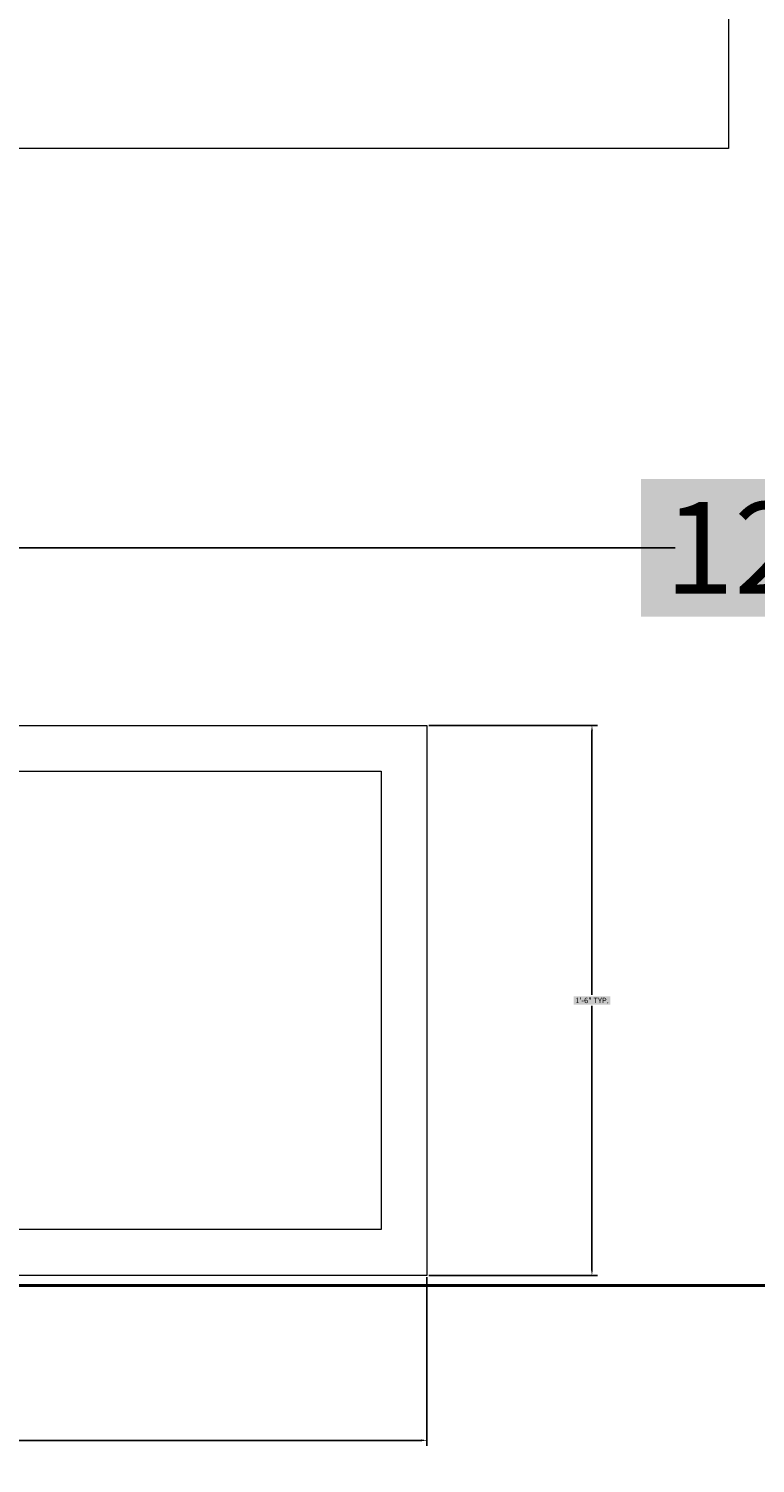
# Model space of a CAD drawing. Units: inches. Extents: x -301 to 715, y -607 to 364.
# Tile 70 of 141: x -147 to -123, y -73 to -26. Entities that reach past the tile are written whole.
import ezdxf

# ---------------------------------------------------------------- set-up
doc = ezdxf.new("R2010")
doc.units = ezdxf.units.IN
doc.header["$MEASUREMENT"] = 0
for name, color, linetype, lineweight in [('A-ANNO-DIMS', 2, 'Continuous', 18), ('A-FLOR-CASE', 8, 'Continuous', 18), ('A-FURN', 8, 'Continuous', 18), ('A-WALL', 3, 'Continuous', 40)]:
    doc.layers.add(name, color=color, linetype=linetype, lineweight=lineweight)
doc.styles.get("Standard").update_dxf_attribs({"font": 'arial.ttf'})
doc.dimstyles.get("Standard").update_dxf_attribs({"dimtxt": 0.18, "dimasz": 0.18, "dimexe": 0.18, "dimexo": 0.0625, "dimgap": 0.09, "dimtad": 0, "dimtih": 1, "dimtoh": 1, "dimdec": 1, "dimzin": 0, "dimdsep": 46, "dimlunit": 4, "dimtxsty": 'Standard', "dimcen": 0.09, "dimclrd": 3, "dimclre": 4, "dimclrt": 6, "dimadec": 0, "dimazin": 0, "dimtfac": 1, "dimtdec": 1, "dimtofl": 0, "dimtmove": 0, "dimatfit": 3, "dimfxl": 1, "dimtfill": 2, "dimtfillclr": 51, "dimtolj": 1, "dimtzin": 0, "dimarcsym": 0})

# ---------------------------------------------------------------- blocks, each defined once
blk = doc.blocks.new('Bed - Queen')
for p, q in [((0, -80.00003), (0, 0)), ((59.99999, -80.00003), (0, -80.00003))]:
    blk.add_line(p, q)
blk = doc.blocks.new('Wall Cabinet - 18 x 36 in front')
for p, q in [((17.5, -1.5), (17.5, -16.5)), ((18.5, -16.5), (18.5, -1.5))]:
    blk.add_line(p, q)
blk.add_lwpolyline([(0, -18), (0, 0), (36, 0), (36, -18)], close=True)
for points in [[(17.5, -16.5), (1.5, -16.5), (1.5, -1.5), (17.5, -1.5)], [(18.5, -1.5), (34.5, -1.5), (34.5, -16.5), (18.5, -16.5)]]:
    blk.add_lwpolyline(points)
blk = doc.blocks.new('*D57')
at = {"layer": 'A-ANNO-DIMS', "color": 0, "lineweight": -2, "transparency": 16777216}
for p, q in [((-195.603, -67.255), (-195.603, -42.99)), ((-190.603, -43.17), (-126.098, -43.17)), ((-56.603, -43.17), (-121.109, -43.17)), ((-51.603, -67.255), (-51.603, -42.99))]:
    blk.add_line(p, q, dxfattribs=at)
at = {"layer": 'A-ANNO-DIMS', "color": 0, "transparency": 16777216}
for points in [[(-190.603, -42.336), (-190.603, -44.003), (-195.603, -43.17)], [(-56.603, -42.336), (-56.603, -44.003), (-51.603, -43.17)]]:
    blk.add_solid(points, dxfattribs=at)
at = {"layer": 'Defpoints', "color": 0, "transparency": 16777216}
for p in [(-51.603, -43.17), (-195.603, -67.318), (-51.603, -67.318)]:
    blk.add_point(p, dxfattribs=at)
at = {"layer": 'A-ANNO-DIMS', "color": 0, "transparency": 16777216, "insert": (-123.603, -43.17), "char_height": 3, "attachment_point": 5, "bg_fill": 1, "box_fill_scale": 1.25, "bg_fill_color": 51, "bg_fill_transparency": 0}
blk.add_mtext("\\A1;12'", dxfattribs=at)
blk = doc.blocks.new('*D120')
at = {"layer": 'A-ANNO-DIMS', "color": 4, "lineweight": -2, "transparency": 16777216}
for p, q in [((-170.223, -67.046), (-170.223, -72.563)), ((-134.223, -67.046), (-134.223, -72.563))]:
    blk.add_line(p, q, dxfattribs=at)
at = {"layer": 'A-ANNO-DIMS', "color": 3, "lineweight": -2, "transparency": 16777216}
for p, q in [((-170.043, -72.383), (-153.822, -72.383)), ((-134.403, -72.383), (-150.623, -72.383))]:
    blk.add_line(p, q, dxfattribs=at)
at = {"layer": 'A-ANNO-DIMS', "color": 3, "transparency": 16777216}
for points in [[(-170.043, -72.353), (-170.043, -72.413), (-170.223, -72.383)], [(-134.403, -72.353), (-134.403, -72.413), (-134.223, -72.383)]]:
    blk.add_solid(points, dxfattribs=at)
at = {"layer": 'Defpoints', "color": 0, "transparency": 16777216}
for p in [(-170.223, -66.983), (-134.223, -66.983), (-134.223, -72.383)]:
    blk.add_point(p, dxfattribs=at)
at = {"layer": 'A-ANNO-DIMS', "color": 6, "transparency": 16777216, "insert": (-152.223, -72.383), "char_height": 0.18, "attachment_point": 5, "bg_fill": 1, "box_fill_scale": 1.25, "bg_fill_color": 51, "bg_fill_transparency": 0}
blk.add_mtext('\\A1;WALL CABINET 3\'-0" TYP.', dxfattribs=at)
blk = doc.blocks.new('*D121')
at = {"layer": 'A-ANNO-DIMS', "color": 4, "lineweight": -2, "transparency": 16777216}
for p, q in [((-134.16, -48.983), (-128.643, -48.983)), ((-134.16, -66.983), (-128.643, -66.983))]:
    blk.add_line(p, q, dxfattribs=at)
at = {"layer": 'A-ANNO-DIMS', "color": 3, "lineweight": -2, "transparency": 16777216}
for p, q in [((-128.823, -49.163), (-128.823, -57.801)), ((-128.823, -66.803), (-128.823, -58.165))]:
    blk.add_line(p, q, dxfattribs=at)
at = {"layer": 'A-ANNO-DIMS', "color": 3, "transparency": 16777216}
for points in [[(-128.853, -49.163), (-128.793, -49.163), (-128.823, -48.983)], [(-128.853, -66.803), (-128.793, -66.803), (-128.823, -66.983)]]:
    blk.add_solid(points, dxfattribs=at)
at = {"layer": 'Defpoints', "color": 0, "transparency": 16777216}
for p in [(-134.223, -48.983), (-128.823, -48.983), (-134.223, -66.983)]:
    blk.add_point(p, dxfattribs=at)
at = {"layer": 'A-ANNO-DIMS', "color": 6, "transparency": 16777216, "insert": (-128.823, -57.983), "char_height": 0.18, "attachment_point": 5, "bg_fill": 1, "box_fill_scale": 1.25, "bg_fill_color": 51, "bg_fill_transparency": 0}
blk.add_mtext('\\A1;1\'-6" TYP.', dxfattribs=at)
blk = doc.blocks.new('*D151')
at = {"layer": 'A-ANNO-DIMS', "color": 4, "lineweight": -2, "transparency": 16777216}
for p, q in [((-204.603, -223.755), (-204.603, 359.612)), ((-45.603, -214.755), (-45.603, 359.612))]:
    blk.add_line(p, q, dxfattribs=at)
at = {"layer": 'A-ANNO-DIMS', "color": 3, "lineweight": -2, "transparency": 16777216}
for p, q in [((-204.423, 359.432), (-125.494, 359.432)), ((-45.783, 359.432), (-124.713, 359.432))]:
    blk.add_line(p, q, dxfattribs=at)
at = {"layer": 'A-ANNO-DIMS', "color": 3, "transparency": 16777216}
for points in [[(-204.423, 359.462), (-204.423, 359.402), (-204.603, 359.432)], [(-45.783, 359.462), (-45.783, 359.402), (-45.603, 359.432)]]:
    blk.add_solid(points, dxfattribs=at)
at = {"layer": 'Defpoints', "color": 0, "transparency": 16777216}
for p in [(-45.603, 359.432), (-45.603, -214.818), (-204.603, -223.818)]:
    blk.add_point(p, dxfattribs=at)
at = {"layer": 'A-ANNO-DIMS', "color": 6, "transparency": 16777216, "insert": (-125.103, 359.432), "char_height": 0.18, "attachment_point": 5, "bg_fill": 1, "box_fill_scale": 1.25, "bg_fill_color": 51, "bg_fill_transparency": 0}
blk.add_mtext('\\A1;13\'-3"', dxfattribs=at)

msp = doc.modelspace()

# ---------------------------------------------------------------- linework, layer by layer
at = {"layer": 'A-WALL'}
msp.add_line((-195.603, -67.318), (-51.603, -67.318), dxfattribs=at)

# ---------------------------------------------------------------- block references
at = {"layer": 'A-FLOR-CASE'}
msp.add_blockref('Wall Cabinet - 18 x 36 in front', (-170.223, -48.983), dxfattribs=at)
at = {"layer": 'A-FURN', "xscale": 0.8856750462000775, "yscale": 0.8856750462000775, "zscale": 0.8856750462000775, "rotation": 90}
msp.add_blockref('Bed - Queen', (-195.207, -30.095), dxfattribs=at)

# ---------------------------------------------------------------- dimensions: what is measured, and where the dimension line sits
at = {"layer": 'A-ANNO-DIMS'}
for base, p1, p2, override, picture, middle in [((-45.603, 359.432), (-204.603, -223.818), (-45.603, -214.818), {"dimdec": 1, "dimlfac": 1, "dimrnd": 0, "dimzin": 1, "dimdsep": 46, "dimlunit": 4, "dimfrac": 2}, '*D151', (-125.103, 359.432)), ((-51.603, -43.17), (-195.603, -67.318), (-51.603, -67.318), {"dimtxt": 3, "dimasz": 5, "dimclrd": 0, "dimclre": 0, "dimclrt": 0}, '*D57', (-123.603, -43.17))]:
    dim = msp.add_linear_dim(base=base, p1=p1, p2=p2, dimstyle='Standard', override=override, dxfattribs=at)
    dim.commit()
    dim.dimension.update_dxf_attribs({"geometry": picture, "text_midpoint": middle})
dim = msp.add_linear_dim(base=(-128.823, -48.983), p1=(-134.223, -66.983), p2=(-134.223, -48.983), angle=90, text='<> TYP.', dimstyle='Standard', override={"dimdec": 1, "dimlfac": 1, "dimrnd": 0, "dimzin": 1, "dimdsep": 46, "dimlunit": 4, "dimfrac": 2}, dxfattribs=at)
dim.commit()
dim.dimension.update_dxf_attribs({"geometry": '*D121', "text_midpoint": (-128.823, -57.983)})
dim = msp.add_linear_dim(base=(-134.223, -72.383), p1=(-170.223, -66.983), p2=(-134.223, -66.983), text='WALL CABINET <> TYP.', dimstyle='Standard', override={"dimdec": 1, "dimlfac": 1, "dimrnd": 0, "dimzin": 1, "dimdsep": 46, "dimlunit": 4, "dimfrac": 2}, dxfattribs=at)
dim.commit()
dim.dimension.update_dxf_attribs({"geometry": '*D120', "text_midpoint": (-152.223, -72.383)})

doc.saveas('drawing.dxf')
